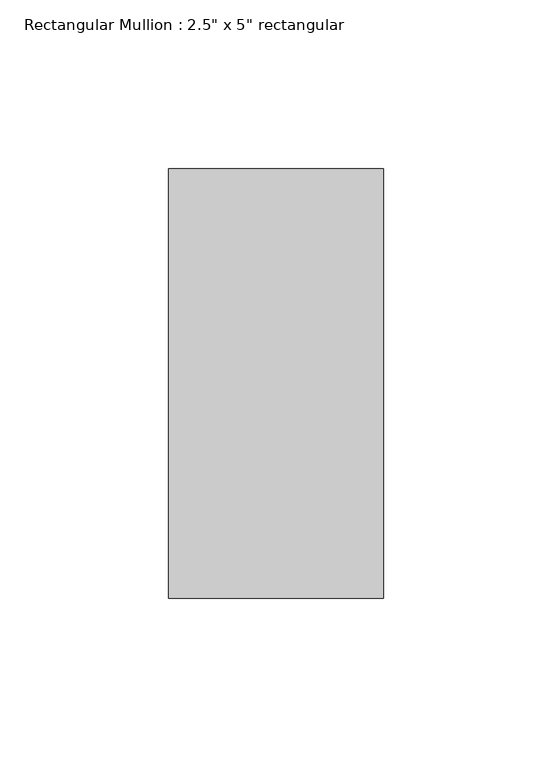
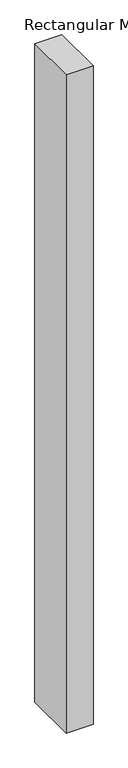
"""IFC4 building model written with IfcOpenShell, lengths in millimetres: member geometry."""

from ifc_helpers import new_model, si_unit, frame, origin, place, context, project, spatial, polyline, outline, extrude, source, transform, mapped, element, save


def member_dc48f745(model_context):
    return source(origin(), model_context, "Body", "SweptSolid", [
        extrude(outline(polyline([(31.75, 63.5), (31.75, -63.5), (-31.75, -63.5), (-31.75, 63.5), (31.75, 63.5)])), frame((0.0, 0.0, -1636.844519), z_axis=(0.0, 0.0, 1.0), x_axis=(1.0, 0.0, 0.0)), (0.0, 0.0, 1.0), 1636.844519),
    ])


if __name__ == "__main__":
    model = new_model("IFC4")
    model_context = context("Model", 3, world=origin())
    ifc_project = project(units=[si_unit("LENGTHUNIT", "METRE", prefix="MILLI")], contexts=[model_context])
    site = spatial("IfcSite", under=ifc_project)
    building = spatial("IfcBuilding", under=site)
    placement = place(None, origin())
    member_shape = member_dc48f745(model_context)
    element("IfcMember", 1, ObjectType="Rectangular Mullion : 2.5\" x 5\" rectangular", at=placement, inside=building, context=model_context, shape_type="MappedRepresentation", body=[
        mapped(member_shape, transform((0.0, 0.0, 0.0), x_axis=(1.0, 0.0, 0.0), y_axis=(0.0, 1.0, 0.0), z_axis=(0.0, 0.0, 1.0))),
    ])
    save(model, "model.ifc")

# Revit data of these elements
# Type "Rectangular Mullion : 2.5\" x 5\" rectangular"
#   built-in parameter 1007304 = 0.416667 (stored number, unit not read)
#   built-in parameter 1007301 = 0.104167 (stored number, unit not read)
#   built-in parameter 1007300 = 0.104167 (stored number, unit not read)
# Element 1 (IfcMember, "Rectangular Mullion : 2.5\" x 5\" rectangular")
#   Materials on its faces: "Aluminum"
# Materials
#   "Aluminum": class "Metal", colour RGB 247 247 247, transparency 0, Description = "Aluminum 6061", Cost = 0
